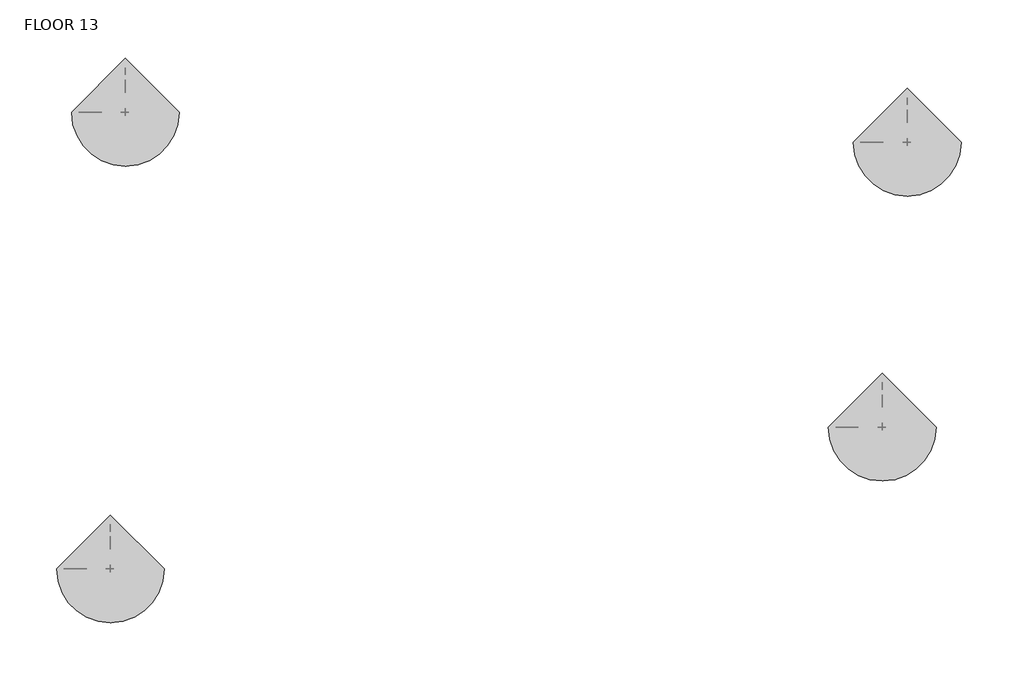
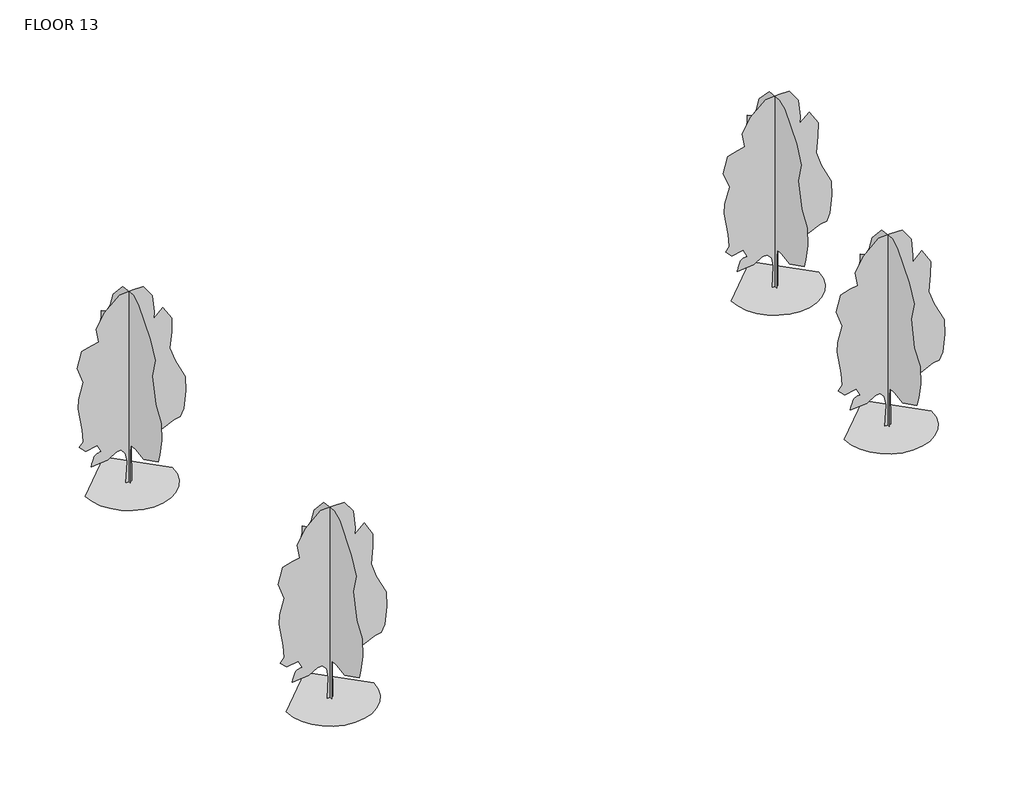
# One storey: 4 geographic elements.
"""IFC4 building model written with IfcOpenShell, lengths in millimetres."""

from ifc_helpers import new_model, si_unit, origin, place, context, project, spatial, transform, mapped, element, save
from components import rpc_tree_deciduous_red_ash_25_14781bec

model = new_model("IFC4")

# Units and contexts
model_context = context("Model", 3, world=origin())
ifc_project = project(units=[si_unit("LENGTHUNIT", "METRE", prefix="MILLI")], contexts=[model_context])

# Site, building, storey
site = spatial("IfcSite", under=ifc_project)
building = spatial("IfcBuilding", under=site)
storey = spatial("IfcBuildingStorey", under=building, Name="FLOOR 13", Elevation=-152.4)

# Geographic elements
placement = place(None, origin())
rpc_tree_deciduous_red_ash_25_shape = rpc_tree_deciduous_red_ash_25_14781bec(model_context)
element("IfcGeographicElement", 1, ObjectType="RPC Tree - Deciduous : Red Ash - 25'", at=placement, inside=storey, context=model_context, shape_type="MappedRepresentation", body=[
    mapped(rpc_tree_deciduous_red_ash_25_shape, transform((6683.0862669, -2285.2593836, -152.4), x_axis=(1.0, 0.0, 0.0), y_axis=(0.0, 1.0, 0.0), z_axis=(0.0, 0.0, 1.0))),
])
element("IfcGeographicElement", 2, ObjectType="RPC Tree - Deciduous : Red Ash - 25'", at=placement, inside=storey, context=model_context, shape_type="MappedRepresentation", body=[
    mapped(rpc_tree_deciduous_red_ash_25_shape, transform((7445.0862669, 6415.8281164, -152.4), x_axis=(1.0, 0.0, 0.0), y_axis=(0.0, 1.0, 0.0), z_axis=(0.0, 0.0, 1.0))),
])
element("IfcGeographicElement", 3, ObjectType="RPC Tree - Deciduous : Red Ash - 25'", at=placement, inside=storey, context=model_context, shape_type="MappedRepresentation", body=[
    mapped(rpc_tree_deciduous_red_ash_25_shape, transform((-16888.1137331, -6615.9593836, -152.4), x_axis=(1.0, 0.0, 0.0), y_axis=(0.0, 1.0, 0.0), z_axis=(0.0, 0.0, 1.0))),
])
element("IfcGeographicElement", 4, ObjectType="RPC Tree - Deciduous : Red Ash - 25'", at=placement, inside=storey, context=model_context, shape_type="MappedRepresentation", body=[
    mapped(rpc_tree_deciduous_red_ash_25_shape, transform((-16430.9137331, 7330.2281164, -152.4), x_axis=(1.0, 0.0, 0.0), y_axis=(0.0, 1.0, 0.0), z_axis=(0.0, 0.0, 1.0))),
])

save(model, "model.ifc")

# Revit data of these elements
# Type "RPC Tree - Deciduous : Red Ash - 25'"
#   built-in parameter 1005198 = "{2, 15},{22, RPC-8-G3GR-497X-PHW5-6},{1, 0},{1, 0},{2, 37},{1, 8},{5, Color},{1, 0},{1, 0},{3, 0.8},{3, 0.8},{3, 0.8},{1, 8},{7, BBoxMin},{1, 0},{1, 0},{1, 0},{1, 0},{1, 0},{1, 8},{7, BBoxMax},{1, 0},{1, 0},{1, 0},{1, 0},{1, 0},{2, 11},{9, RPCTypeId},{1, 0},{1, 0},{22, RPC-8-G3GR-497X-PHW5-6},{1, 6},{14, RPCPlantHeight},{1, 0},{1, 0},{2, 25},{2, 11},{7, keyword},{1, 0},{1, 0},{78, :Geometry:RPC:Red Ash:red ash:frainus pennsylvanica:frene rouge:deciduous:tree},{2, 11},{8, category},{1, 0},{1, 0},{16, :Trees [General]},{2, 11},{12, LocalizedUID},{1, 0},{1, 0},{7, Red Ash},{2, 14},{6, Height},{1, 0},{1, 0},{2, 25},{1, 2},{16, Cast Reflections},{1, 0},{1, 0},{1, 0},{1, 2},{6, Jitter},{1, 0},{1, 0},{1, 1},{1, 2},{9, Billboard},{1, 0},{1, 0},{1, 0},{1, 2},{12, Cast Shadows},{1, 0},{1, 0},{1, 1},{1, 2},{20, Apply Filter Effects},{1, 0},{1, 0},{1, 0},{2, 11},{28, Apply Filter Effects-Text-FC},{1, 0},{1, 0},{4, None},{2, 11},{20, AdvancedUIDefinition},{1, 0},{1, 0},{0, },{2, 11},{10, AssetLibID},{1, 0},{1, 0},{36, 4D3F6E72-3F99-4203-98E9-AF80B3C7A7A4},{2, 11},{10, BaseSchema},{1, 0},{1, 0},{9, RPCSchema},{2, 11},{12, ExchangeGUID},{1, 0},{1, 0},{0, },{1, 2},{6, Hidden},{1, 0},{1, 0},{1, 0},{1, 4},{11, RPCCategory},{1, 0},{1, 0},{1, 0},{2, 11},{8, RPCImage},{1, 0},{1, 0},{0, },{1, 4},{13, SchemaVersion},{1, 0},{1, 0},{1, 4},{2, 11},{12, UIDefinition},{1, 0},{1, 0},{0, },{2, 11},{6, UIName},{1, 0},{1, 0},{22, RPC-8-G3GR-497X-PHW5-6},{2, 11},{11, VersionGUID},{1, 0},{1, 0},{9, RPCSchema},{2, 11},{9, assettype},{1, 0},{1, 0},{11, RPCGeometry},{2, 11},{11, description},{1, 0},{1, 0},{0, },{2, 11},{9, localname},{1, 0},{1, 0},{3, RPC},{2, 11},{9, localtype},{1, 0},{1, 0},{3, RPC},{1, 4},{8, revision},{1, 0},{1, 0},{1, 1},{2, 11},{9, thumbnail},{1, 0},{1, 0},{0, },{1, 4},{7, version},{1, 0},{1, 0},{1, 1},{1, 2},{20, RPC_Cast Reflections},{1, 0},{1, 0},{1, 1},{1, 2},{10, RPC_Jitter},{1, 0},{1, 0},{1, 1},{1, 2},{13, RPC_Billboard},{1, 0},{1, 0},{1, 0},{1, 2},{16, RPC_Cast Shadows},{1, 0},{1, 0},{1, 1},{21, assetlibrary_base.fbx},{1, 5},"
#   built-in parameter 1005195 = "RPC-8-G3GR-497X-PHW5-6"
#   Type Comments = "Red Maple"
#   Assembly Code = "G2050500"
#   Height = 25' - 0"
#   Default Elevation = 0
# Elements 1, 2, 3, 4 (IfcGeographicElement, "RPC Tree - Deciduous : Red Ash - 25'")
#   Phase Created = New Construction
